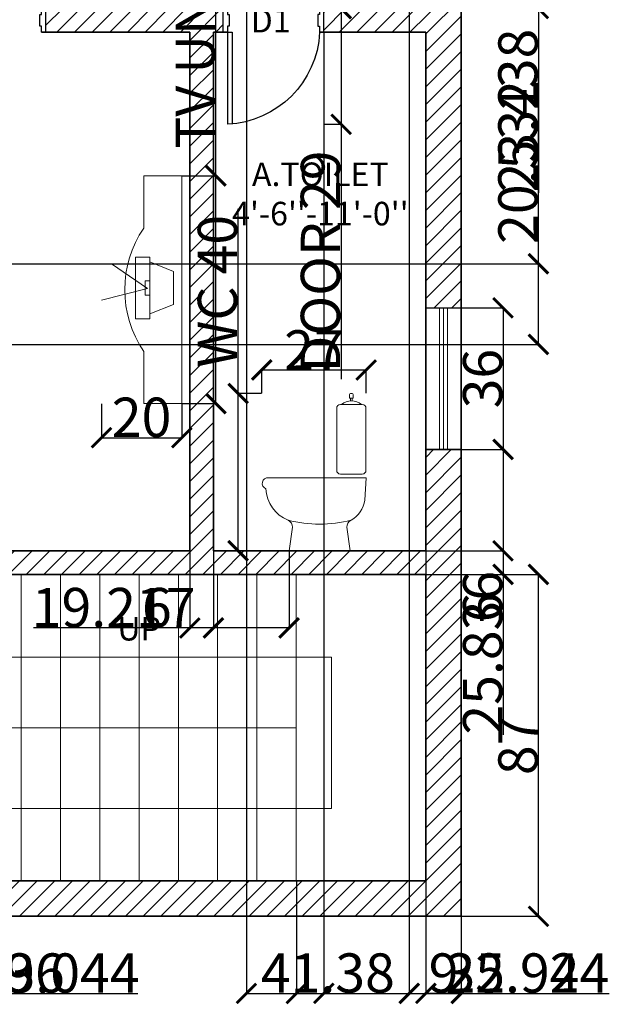
# Model space of a CAD drawing. Units: inches. Extents: x 90933 to 91345, y 21207 to 21646.
# Tile 2 of 4: x 91195 to 91345, y 21207 to 21458. Entities that reach past the tile are written whole.
import ezdxf

# ---------------------------------------------------------------- set-up
doc = ezdxf.new("R2010")
doc.units = ezdxf.units.IN
for name, color, linetype, lineweight in [('A-ANNO-DIMS', 2, 'Continuous', 18), ('A-ANNO-TEXT', 7, 'Continuous', 18), ('A-AREA-IDEN', 7, 'Continuous', 25), ('A-FLOR-FIXT', 9, 'Continuous', 18), ('A-WALL-PATT', 8, 'Continuous', 13), ('B-FURNITURE', 9, 'Continuous', 18), ('Doors', 34, 'Continuous', 25), ('Steps', 50, 'Continuous', 18), ('Ven', 120, 'Continuous', 18), ('Walls', 7, 'Continuous', 35)]:
    doc.layers.add(name, color=color, linetype=linetype, lineweight=lineweight)
doc.styles.get("Standard").update_dxf_attribs({"font": 'arial.ttf'})
doc.dimstyles.get("Standard").update_dxf_attribs({"dimtxt": 10, "dimasz": 5, "dimexe": 0.18, "dimexo": 0.0625, "dimgap": 0.09, "dimtad": 1, "dimdec": 1, "dimzin": 0, "dimdsep": 46, "dimlunit": 4, "dimtxsty": 'Standard', "dimblk": 'ARCHTICK', "dimcen": 0.09, "dimadec": 0, "dimazin": 0, "dimtfac": 1, "dimtdec": 1, "dimtofl": 0, "dimtmove": 0, "dimatfit": 3, "dimldrblk": 'NONE', "dimfxl": 1, "dimtolj": 1, "dimtzin": 0, "dimarcsym": 0})

# ---------------------------------------------------------------- blocks, each defined once
blk = doc.blocks.new('toil-el-1')
at = {"color": 0, "linetype": 'ByBlock'}
for p, q in [((-0.0048, 1.026), (-0.0048, 1.002)), ((-0.0048, 1.002), (0.0192, 1.002)), ((0.0012, 1.032), (0.0132, 1.032)), ((0.0012, 1.002), (0.0012, 0.984)), ((0.0132, 1.002), (0.0132, 0.984)), ((0.0192, 1.026), (0.0192, 1.002)), ((-0.0888, 0.936), (-0.0888, 0.528)), ((0.0792, 0.96), (-0.0648, 0.96)), ((0.1032, 0.936), (0.1032, 0.528)), ((0.1047, 0.48), (-0.543, 0.48)), ((0.0792, 0.504), (-0.0648, 0.504)), ((0.0966, 0.3327), (0.1047, 0.48)), ((-0.3785, 0.1552), (-0.4013, 0)), ((-0.0228, 0.1552), (0, 0)), ((-0.4013, 0), (0, 0))]:
    blk.add_line(p, q, dxfattribs=at)
for centre, radius, start, end in [((0.0084, 0.8817), 0.1023, 49.95059, 130.04941), ((0.0012, 1.026), 0.006, 90, 180), ((0.0132, 1.026), 0.006, 0, 90), ((-0.0648, 0.936), 0.024, 90, 180), ((0.0792, 0.936), 0.024, 0, 90), ((-0.0648, 0.528), 0.024, 180, 270), ((0.0792, 0.528), 0.024, 270, 0), ((-0.5394, 0.4428), 0.0373, 84.42239, 249.75453), ((-0.3163, 0.4187), 0.2362, 182.64484, 247.30718), ((-0.0919, 0.3648), 0.1912, 300.87439, 350.34418), ((-0.4257, 0.1572), 0.0472, 357.60433, 67.30718), ((-0.2006, 1.0367), 0.8612, 256.10247, 283.89753), ((0.0244, 0.1572), 0.0472, 112.69282, 182.39567)]:
    blk.add_arc(centre, radius, start, end, dxfattribs=at)
blk = doc.blocks.new('AP0B05')
for p, q in [((35, 100), (35, 880)), ((75, 100), (75, 878.9))]:
    blk.add_line(p, q)
for points in [[(0, 100), (0, -100), (35, -100), (35, -50), (50, -50), (50, 50), (35, 50), (35, 100)], [(850, 100), (850, -100), (815, -100), (815, -50), (800, -50), (800, 50), (815, 50), (815, 100)]]:
    blk.add_lwpolyline(points, close=True)
blk.add_lwpolyline([(35, 100), (75, 100)])
blk.add_arc((-2.4, 62.6), 818.3, 2.62122, 87.37878)
blk = doc.blocks.new('banghe81')
for p, q in [((-500, 3000), (0, 3000)), ((-500, 2312), (-500, 3000)), ((0, 3000), (0, 0)), ((-925, 1843), (-450, 1517)), ((-607, 1930), (-419, 1930)), ((-607, 1117), (-607, 1930)), ((-419, 1930), (-419, 1117)), ((-107, 1742), (-419, 1867)), ((-107, 1305), (-107, 1742)), ((-482, 1617), (-482, 1430)), ((-419, 1617), (-482, 1617)), ((-450, 1517), (-1057, 1361)), ((-482, 1430), (-419, 1430)), ((-419, 1180), (-107, 1305)), ((-419, 1117), (-607, 1117)), ((-500, 0), (-500, 688)), ((0, 0), (-500, 0)), ((-500, 0), (-500, 0))]:
    blk.add_line(p, q)
blk.add_arc((695, 1500), 1445, 145.7945, 214.2055)
blk = doc.blocks.new('_ArchTick')
at = {"color": 0, "linetype": 'ByBlock', "const_width": 0.15}
blk.add_lwpolyline([(-0.5, -0.5), (0.5, 0.5)], dxfattribs=at)
blk = doc.blocks.new('*D22')
at = {"layer": 'A-ANNO-DIMS', "color": 0, "lineweight": -2, "transparency": 16777216}
for p, q in [((91272.22, 21460.62), (91276.76, 21460.62)), ((91276.58, 21460.62), (91276.58, 21431.16)), ((91272.22, 21431.16), (91276.76, 21431.16)), ((91276.58, 21431.16), (91276.58, 21366.34))]:
    blk.add_line(p, q, dxfattribs=at)
at = {"layer": 'Defpoints', "color": 0, "transparency": 16777216}
for p in [(91272.16, 21460.62), (91272.16, 21431.16), (91276.58, 21431.16)]:
    blk.add_point(p, dxfattribs=at)
at = {"layer": 'A-ANNO-DIMS', "color": 0, "lineweight": -2, "transparency": 16777216, "xscale": 5, "yscale": 5, "zscale": 5}
for p, rotation in [((91276.58, 21460.62), 90), ((91276.58, 21431.16), 270)]:
    blk.add_blockref('_ArchTick', p, dxfattribs=dict(at, rotation=rotation))
at = {"layer": 'A-ANNO-DIMS', "color": 0, "transparency": 16777216, "insert": (91271.31, 21396.25), "char_height": 10, "attachment_point": 5, "rotation": 90}
blk.add_mtext('\\A1;DOOR 29', dxfattribs=at)
blk = doc.blocks.new('_None')
blk = doc.blocks.new('*D32')
at = {"layer": 'A-ANNO-DIMS', "color": 0, "lineweight": -2, "transparency": 16777216}
for p, q in [((91250.38, 21362.65), (91250.38, 21409.68)), ((91256.32, 21362.65), (91250.2, 21362.65)), ((91250.38, 21322.62), (91250.38, 21362.65)), ((91256.32, 21322.62), (91250.2, 21322.62))]:
    blk.add_line(p, q, dxfattribs=at)
at = {"layer": 'Defpoints', "color": 0, "transparency": 16777216}
for p in [(91250.38, 21362.65), (91256.38, 21362.65), (91256.38, 21322.62)]:
    blk.add_point(p, dxfattribs=at)
at = {"layer": 'A-ANNO-DIMS', "color": 0, "lineweight": -2, "transparency": 16777216, "xscale": 5, "yscale": 5, "zscale": 5}
for p, rotation in [((91250.38, 21362.65), 90), ((91250.38, 21322.62), 270)]:
    blk.add_blockref('_ArchTick', p, dxfattribs=dict(at, rotation=rotation))
at = {"layer": 'A-ANNO-DIMS', "color": 0, "transparency": 16777216, "insert": (91245.12, 21388.67), "char_height": 10, "attachment_point": 5, "rotation": 90}
blk.add_mtext('\\A1;WC 40', dxfattribs=at)
blk = doc.blocks.new('*D33')
at = {"layer": 'A-ANNO-DIMS', "color": 0, "lineweight": -2, "transparency": 16777216}
for p, q in [((91256.38, 21362.71), (91256.38, 21368.83)), ((91256.38, 21368.65), (91282.95, 21368.65)), ((91282.95, 21362.71), (91282.95, 21368.83))]:
    blk.add_line(p, q, dxfattribs=at)
at = {"layer": 'Defpoints', "color": 0, "transparency": 16777216}
for p in [(91282.95, 21368.65), (91256.38, 21362.65), (91282.95, 21362.65)]:
    blk.add_point(p, dxfattribs=at)
at = {"layer": 'A-ANNO-DIMS', "color": 0, "lineweight": -2, "transparency": 16777216, "xscale": 5, "yscale": 5, "zscale": 5, "rotation": 180}
blk.add_blockref('_ArchTick', (91256.38, 21368.65), dxfattribs=at)
at = {"layer": 'A-ANNO-DIMS', "color": 0, "lineweight": -2, "transparency": 16777216, "xscale": 5, "yscale": 5, "zscale": 5}
blk.add_blockref('_ArchTick', (91282.95, 21368.65), dxfattribs=at)
at = {"layer": 'A-ANNO-DIMS', "color": 0, "transparency": 16777216, "insert": (91269.66, 21373.76), "char_height": 10, "attachment_point": 5}
blk.add_mtext('\\A1;27', dxfattribs=at)
blk = doc.blocks.new('*D36')
at = {"layer": 'A-ANNO-DIMS', "color": 0, "lineweight": -2, "transparency": 16777216}
for p, q in [((91244.73, 21418.04), (91244.73, 21496.03)), ((91236.1, 21418.04), (91244.91, 21418.04)), ((91244.73, 21360.1), (91244.73, 21418.04)), ((91236.1, 21360.1), (91244.91, 21360.1))]:
    blk.add_line(p, q, dxfattribs=at)
at = {"layer": 'Defpoints', "color": 0, "transparency": 16777216}
for p in [(91236.04, 21418.04), (91244.73, 21418.04), (91236.04, 21360.1)]:
    blk.add_point(p, dxfattribs=at)
at = {"layer": 'A-ANNO-DIMS', "color": 0, "lineweight": -2, "transparency": 16777216, "xscale": 5, "yscale": 5, "zscale": 5}
for p, rotation in [((91244.73, 21418.04), 90), ((91244.73, 21360.1), 270)]:
    blk.add_blockref('_ArchTick', p, dxfattribs=dict(at, rotation=rotation))
at = {"layer": 'A-ANNO-DIMS', "color": 0, "transparency": 16777216, "insert": (91239.53, 21459.53), "char_height": 10, "attachment_point": 5, "rotation": 90}
blk.add_mtext('\\A1;TV UNIT 58', dxfattribs=at)
blk = doc.blocks.new('*D37')
at = {"layer": 'A-ANNO-DIMS', "color": 0, "lineweight": -2, "transparency": 16777216}
for p, q in [((91215.62, 21360.04), (91215.62, 21351.23)), ((91236.04, 21360.04), (91236.04, 21351.23)), ((91215.62, 21351.41), (91236.04, 21351.41))]:
    blk.add_line(p, q, dxfattribs=at)
at = {"layer": 'Defpoints', "color": 0, "transparency": 16777216}
for p in [(91215.62, 21360.1), (91236.04, 21360.1), (91236.04, 21351.41)]:
    blk.add_point(p, dxfattribs=at)
at = {"layer": 'A-ANNO-DIMS', "color": 0, "lineweight": -2, "transparency": 16777216, "xscale": 5, "yscale": 5, "zscale": 5, "rotation": 180}
blk.add_blockref('_ArchTick', (91215.62, 21351.41), dxfattribs=at)
at = {"layer": 'A-ANNO-DIMS', "color": 0, "lineweight": -2, "transparency": 16777216, "xscale": 5, "yscale": 5, "zscale": 5}
blk.add_blockref('_ArchTick', (91236.04, 21351.41), dxfattribs=at)
at = {"layer": 'A-ANNO-DIMS', "color": 0, "transparency": 16777216, "insert": (91225.83, 21356.61), "char_height": 10, "attachment_point": 5}
blk.add_mtext('\\A1;20', dxfattribs=at)
blk = doc.blocks.new('*D39')
at = {"layer": 'A-ANNO-DIMS', "color": 0, "lineweight": -2, "transparency": 16777216}
for p, q in [((91298.16, 21348.45), (91317.91, 21348.45)), ((91317.73, 21348.45), (91317.73, 21322.62)), ((91298.16, 21322.62), (91317.91, 21322.62)), ((91317.73, 21322.62), (91317.73, 21275.76))]:
    blk.add_line(p, q, dxfattribs=at)
at = {"layer": 'Defpoints', "color": 0, "transparency": 16777216}
for p in [(91298.1, 21348.45), (91298.1, 21322.62), (91317.73, 21322.62)]:
    blk.add_point(p, dxfattribs=at)
at = {"layer": 'A-ANNO-DIMS', "color": 0, "lineweight": -2, "transparency": 16777216, "xscale": 5, "yscale": 5, "zscale": 5}
for p, rotation in [((91317.73, 21348.45), 90), ((91317.73, 21322.62), 270)]:
    blk.add_blockref('_ArchTick', p, dxfattribs=dict(at, rotation=rotation))
at = {"layer": 'A-ANNO-DIMS', "color": 0, "transparency": 16777216, "insert": (91312.53, 21296.69), "char_height": 10, "attachment_point": 5, "rotation": 90}
blk.add_mtext('\\A1;25.836', dxfattribs=at)
blk = doc.blocks.new('*D40')
at = {"layer": 'A-ANNO-DIMS', "color": 0, "lineweight": -2, "transparency": 16777216}
for p, q in [((91298.16, 21384.45), (91317.91, 21384.45)), ((91317.73, 21384.45), (91317.73, 21348.45)), ((91298.16, 21348.45), (91317.91, 21348.45))]:
    blk.add_line(p, q, dxfattribs=at)
at = {"layer": 'Defpoints', "color": 0, "transparency": 16777216}
for p in [(91298.1, 21384.45), (91298.1, 21348.45), (91317.73, 21348.45)]:
    blk.add_point(p, dxfattribs=at)
at = {"layer": 'A-ANNO-DIMS', "color": 0, "lineweight": -2, "transparency": 16777216, "xscale": 5, "yscale": 5, "zscale": 5}
for p, rotation in [((91317.73, 21384.45), 90), ((91317.73, 21348.45), 270)]:
    blk.add_blockref('_ArchTick', p, dxfattribs=dict(at, rotation=rotation))
at = {"layer": 'A-ANNO-DIMS', "color": 0, "transparency": 16777216, "insert": (91312.53, 21366.45), "char_height": 10, "attachment_point": 5, "rotation": 90}
blk.add_mtext('\\A1;36', dxfattribs=at)
blk = doc.blocks.new('*D41')
at = {"layer": 'A-ANNO-DIMS', "color": 0, "lineweight": -2, "transparency": 16777216}
for p, q in [((91166.1, 21592.55), (91166.1, 21209.81)), ((91179.14, 21592.55), (91179.14, 21209.81)), ((91166.1, 21209.99), (91179.14, 21209.99)), ((91179.14, 21209.99), (91224.86, 21209.99))]:
    blk.add_line(p, q, dxfattribs=at)
at = {"layer": 'Defpoints', "color": 0, "transparency": 16777216}
for p in [(91166.1, 21592.62), (91179.14, 21592.62), (91179.14, 21209.99)]:
    blk.add_point(p, dxfattribs=at)
at = {"layer": 'A-ANNO-DIMS', "color": 0, "lineweight": -2, "transparency": 16777216, "xscale": 5, "yscale": 5, "zscale": 5, "rotation": 180}
blk.add_blockref('_ArchTick', (91166.1, 21209.99), dxfattribs=at)
at = {"layer": 'A-ANNO-DIMS', "color": 0, "lineweight": -2, "transparency": 16777216, "xscale": 5, "yscale": 5, "zscale": 5}
blk.add_blockref('_ArchTick', (91179.14, 21209.99), dxfattribs=at)
at = {"layer": 'A-ANNO-DIMS', "color": 0, "transparency": 16777216, "insert": (91204.5, 21215.18), "char_height": 10, "attachment_point": 5}
blk.add_mtext('\\A1;13.044', dxfattribs=at)
blk = doc.blocks.new('*D49')
at = {"layer": 'A-ANNO-DIMS', "color": 0, "lineweight": -2, "transparency": 16777216}
for p, q in [((91160.1, 21460.55), (91160.1, 21209.81)), ((91142.5, 21454.55), (91142.5, 21209.81)), ((91142.5, 21209.99), (91160.1, 21209.99)), ((91160.1, 21209.99), (91205.85, 21209.99))]:
    blk.add_line(p, q, dxfattribs=at)
at = {"layer": 'Defpoints', "color": 0, "transparency": 16777216}
for p in [(91160.1, 21460.62), (91142.5, 21454.62), (91160.1, 21209.99)]:
    blk.add_point(p, dxfattribs=at)
at = {"layer": 'A-ANNO-DIMS', "color": 0, "lineweight": -2, "transparency": 16777216, "xscale": 5, "yscale": 5, "zscale": 5, "rotation": 180}
blk.add_blockref('_ArchTick', (91142.5, 21209.99), dxfattribs=at)
at = {"layer": 'A-ANNO-DIMS', "color": 0, "lineweight": -2, "transparency": 16777216, "xscale": 5, "yscale": 5, "zscale": 5}
blk.add_blockref('_ArchTick', (91160.1, 21209.99), dxfattribs=at)
at = {"layer": 'A-ANNO-DIMS', "color": 0, "transparency": 16777216, "insert": (91185.47, 21215.18), "char_height": 10, "attachment_point": 5}
blk.add_mtext('\\A1;17.596', dxfattribs=at)
blk = doc.blocks.new('*D51')
at = {"layer": 'A-ANNO-DIMS', "color": 0, "lineweight": -2, "transparency": 16777216}
for p, q in [((91272.16, 21454.54), (91272.16, 21209.81)), ((91298.1, 21454.55), (91298.1, 21209.81)), ((91272.16, 21209.99), (91298.1, 21209.99)), ((91298.1, 21209.99), (91337.15, 21209.99))]:
    blk.add_line(p, q, dxfattribs=at)
at = {"layer": 'Defpoints', "color": 0, "transparency": 16777216}
for p in [(91272.16, 21454.6), (91298.1, 21454.62), (91298.1, 21209.99)]:
    blk.add_point(p, dxfattribs=at)
at = {"layer": 'A-ANNO-DIMS', "color": 0, "lineweight": -2, "transparency": 16777216, "xscale": 5, "yscale": 5, "zscale": 5, "rotation": 180}
blk.add_blockref('_ArchTick', (91272.16, 21209.99), dxfattribs=at)
at = {"layer": 'A-ANNO-DIMS', "color": 0, "lineweight": -2, "transparency": 16777216, "xscale": 5, "yscale": 5, "zscale": 5}
blk.add_blockref('_ArchTick', (91298.1, 21209.99), dxfattribs=at)
at = {"layer": 'A-ANNO-DIMS', "color": 0, "transparency": 16777216, "insert": (91320.13, 21215.18), "char_height": 10, "attachment_point": 5}
blk.add_mtext('\\A1;25.94', dxfattribs=at)
blk = doc.blocks.new('*D54')
at = {"layer": 'A-ANNO-DIMS', "color": 0, "lineweight": -2, "transparency": 16777216}
for p, q in [((91298.1, 21238.55), (91298.1, 21209.81)), ((91307.1, 21229.55), (91307.1, 21209.81)), ((91307.1, 21209.99), (91298.1, 21209.99))]:
    blk.add_line(p, q, dxfattribs=at)
at = {"layer": 'Defpoints', "color": 0, "transparency": 16777216}
for p in [(91298.1, 21238.62), (91307.1, 21229.62), (91298.1, 21209.99)]:
    blk.add_point(p, dxfattribs=at)
at = {"layer": 'A-ANNO-DIMS', "color": 0, "lineweight": -2, "transparency": 16777216, "xscale": 5, "yscale": 5, "zscale": 5, "rotation": 180}
blk.add_blockref('_ArchTick', (91298.1, 21209.99), dxfattribs=at)
at = {"layer": 'A-ANNO-DIMS', "color": 0, "lineweight": -2, "transparency": 16777216, "xscale": 5, "yscale": 5, "zscale": 5}
blk.add_blockref('_ArchTick', (91307.1, 21209.99), dxfattribs=at)
at = {"layer": 'A-ANNO-DIMS', "color": 0, "transparency": 16777216, "insert": (91302.6, 21215.18), "char_height": 10, "attachment_point": 5}
blk.add_mtext('\\A1;9', dxfattribs=at)
blk = doc.blocks.new('*D56')
at = {"layer": 'A-ANNO-DIMS', "color": 0, "lineweight": -2, "transparency": 16777216}
for p, q in [((91265.18, 21238.55), (91265.18, 21209.81)), ((91298.1, 21238.55), (91298.1, 21209.81)), ((91265.18, 21209.99), (91298.1, 21209.99)), ((91298.1, 21209.99), (91344.75, 21209.99))]:
    blk.add_line(p, q, dxfattribs=at)
at = {"layer": 'Defpoints', "color": 0, "transparency": 16777216}
for p in [(91265.18, 21238.62), (91298.1, 21238.62), (91298.1, 21209.99)]:
    blk.add_point(p, dxfattribs=at)
at = {"layer": 'A-ANNO-DIMS', "color": 0, "lineweight": -2, "transparency": 16777216, "xscale": 5, "yscale": 5, "zscale": 5, "rotation": 180}
blk.add_blockref('_ArchTick', (91265.18, 21209.99), dxfattribs=at)
at = {"layer": 'A-ANNO-DIMS', "color": 0, "lineweight": -2, "transparency": 16777216, "xscale": 5, "yscale": 5, "zscale": 5}
blk.add_blockref('_ArchTick', (91298.1, 21209.99), dxfattribs=at)
at = {"layer": 'A-ANNO-DIMS', "color": 0, "transparency": 16777216, "insert": (91323.92, 21215.18), "char_height": 10, "attachment_point": 5}
blk.add_mtext('\\A1;32.924', dxfattribs=at)
blk = doc.blocks.new('*D61')
at = {"layer": 'A-ANNO-DIMS', "color": 0, "lineweight": -2, "transparency": 16777216}
for p, q in [((91326.73, 21395.68), (91326.73, 21442.44)), ((91153.57, 21395.68), (91326.91, 21395.68)), ((91326.73, 21375.15), (91326.73, 21395.68)), ((91153.57, 21375.15), (91326.91, 21375.15))]:
    blk.add_line(p, q, dxfattribs=at)
at = {"layer": 'Defpoints', "color": 0, "transparency": 16777216}
for p in [(91153.51, 21395.68), (91326.73, 21395.68), (91153.51, 21375.15)]:
    blk.add_point(p, dxfattribs=at)
at = {"layer": 'A-ANNO-DIMS', "color": 0, "lineweight": -2, "transparency": 16777216, "xscale": 5, "yscale": 5, "zscale": 5}
for p, rotation in [((91326.73, 21395.68), 90), ((91326.73, 21375.15), 270)]:
    blk.add_blockref('_ArchTick', p, dxfattribs=dict(at, rotation=rotation))
at = {"layer": 'A-ANNO-DIMS', "color": 0, "transparency": 16777216, "insert": (91321.53, 21421.56), "char_height": 10, "attachment_point": 5, "rotation": 90}
blk.add_mtext('\\A1;20.532', dxfattribs=at)
blk = doc.blocks.new('*D62')
at = {"layer": 'A-ANNO-DIMS', "color": 0, "lineweight": -2, "transparency": 16777216}
for p, q in [((91252.49, 21576.95), (91252.49, 21209.81)), ((91293.88, 21576.95), (91293.88, 21209.81)), ((91252.49, 21209.99), (91293.88, 21209.99))]:
    blk.add_line(p, q, dxfattribs=at)
at = {"layer": 'Defpoints', "color": 0, "transparency": 16777216}
for p in [(91252.49, 21577.01), (91293.88, 21577.01), (91293.88, 21209.99)]:
    blk.add_point(p, dxfattribs=at)
at = {"layer": 'A-ANNO-DIMS', "color": 0, "lineweight": -2, "transparency": 16777216, "xscale": 5, "yscale": 5, "zscale": 5, "rotation": 180}
blk.add_blockref('_ArchTick', (91252.49, 21209.99), dxfattribs=at)
at = {"layer": 'A-ANNO-DIMS', "color": 0, "lineweight": -2, "transparency": 16777216, "xscale": 5, "yscale": 5, "zscale": 5}
blk.add_blockref('_ArchTick', (91293.88, 21209.99), dxfattribs=at)
at = {"layer": 'A-ANNO-DIMS', "color": 0, "transparency": 16777216, "insert": (91273.18, 21215.18), "char_height": 10, "attachment_point": 5}
blk.add_mtext('\\A1;41.38', dxfattribs=at)
blk = doc.blocks.new('*D68')
at = {"layer": 'A-ANNO-DIMS', "color": 0, "lineweight": -2, "transparency": 16777216}
for p, q in [((91296.1, 21484.05), (91326.91, 21484.05)), ((91326.73, 21484.05), (91326.73, 21460.62)), ((91298.16, 21460.62), (91326.91, 21460.62)), ((91326.73, 21460.62), (91326.73, 21413.73))]:
    blk.add_line(p, q, dxfattribs=at)
at = {"layer": 'Defpoints', "color": 0, "transparency": 16777216}
for p in [(91296.04, 21484.05), (91298.1, 21460.62), (91326.73, 21460.62)]:
    blk.add_point(p, dxfattribs=at)
at = {"layer": 'A-ANNO-DIMS', "color": 0, "lineweight": -2, "transparency": 16777216, "xscale": 5, "yscale": 5, "zscale": 5}
for p, rotation in [((91326.73, 21484.05), 90), ((91326.73, 21460.62), 270)]:
    blk.add_blockref('_ArchTick', p, dxfattribs=dict(at, rotation=rotation))
at = {"layer": 'A-ANNO-DIMS', "color": 0, "transparency": 16777216, "insert": (91321.53, 21434.67), "char_height": 10, "attachment_point": 5, "rotation": 90}
blk.add_mtext('\\A1;23.438', dxfattribs=at)
blk = doc.blocks.new('*D69')
at = {"layer": 'A-ANNO-DIMS', "color": 0, "lineweight": -2, "transparency": 16777216}
for p, q in [((91244.1, 21322.55), (91244.1, 21302.81)), ((91263.32, 21322.55), (91263.32, 21302.81)), ((91244.1, 21302.99), (91198.35, 21302.99)), ((91263.32, 21302.99), (91244.1, 21302.99))]:
    blk.add_line(p, q, dxfattribs=at)
at = {"layer": 'Defpoints', "color": 0, "transparency": 16777216}
for p in [(91244.1, 21322.62), (91263.32, 21322.62), (91244.1, 21302.99)]:
    blk.add_point(p, dxfattribs=at)
at = {"layer": 'A-ANNO-DIMS', "color": 0, "lineweight": -2, "transparency": 16777216, "xscale": 5, "yscale": 5, "zscale": 5, "rotation": 180}
blk.add_blockref('_ArchTick', (91244.1, 21302.99), dxfattribs=at)
at = {"layer": 'A-ANNO-DIMS', "color": 0, "lineweight": -2, "transparency": 16777216, "xscale": 5, "yscale": 5, "zscale": 5}
blk.add_blockref('_ArchTick', (91263.32, 21302.99), dxfattribs=at)
at = {"layer": 'A-ANNO-DIMS', "color": 0, "transparency": 16777216, "insert": (91218.72, 21308.18), "char_height": 10, "attachment_point": 5}
blk.add_mtext('\\A1;19.217', dxfattribs=at)
blk = doc.blocks.new('*D75')
at = {"layer": 'A-ANNO-DIMS', "color": 0, "lineweight": -2, "transparency": 16777216}
for p, q in [((91298.16, 21316.62), (91326.91, 21316.62)), ((91326.73, 21229.62), (91326.73, 21316.62)), ((91307.16, 21229.62), (91326.91, 21229.62))]:
    blk.add_line(p, q, dxfattribs=at)
at = {"layer": 'Defpoints', "color": 0, "transparency": 16777216}
for p in [(91298.1, 21316.62), (91326.73, 21316.62), (91307.1, 21229.62)]:
    blk.add_point(p, dxfattribs=at)
at = {"layer": 'A-ANNO-DIMS', "color": 0, "lineweight": -2, "transparency": 16777216, "xscale": 5, "yscale": 5, "zscale": 5}
for p, rotation in [((91326.73, 21316.62), 90), ((91326.73, 21229.62), 270)]:
    blk.add_blockref('_ArchTick', p, dxfattribs=dict(at, rotation=rotation))
at = {"layer": 'A-ANNO-DIMS', "color": 0, "transparency": 16777216, "insert": (91321.53, 21273.12), "char_height": 10, "attachment_point": 5, "rotation": 90}
blk.add_mtext('\\A1;87', dxfattribs=at)
blk = doc.blocks.new('*D76')
at = {"layer": 'A-ANNO-DIMS', "color": 0, "lineweight": -2, "transparency": 16777216}
for p, q in [((91298.16, 21322.62), (91317.91, 21322.62)), ((91317.73, 21322.62), (91317.73, 21316.62)), ((91298.16, 21316.62), (91317.91, 21316.62)), ((91317.73, 21316.62), (91317.73, 21304.83))]:
    blk.add_line(p, q, dxfattribs=at)
at = {"layer": 'Defpoints', "color": 0, "transparency": 16777216}
for p in [(91298.1, 21322.62), (91298.1, 21316.62), (91317.73, 21316.62)]:
    blk.add_point(p, dxfattribs=at)
at = {"layer": 'A-ANNO-DIMS', "color": 0, "lineweight": -2, "transparency": 16777216, "xscale": 5, "yscale": 5, "zscale": 5}
for p, rotation in [((91317.73, 21322.62), 90), ((91317.73, 21316.62), 270)]:
    blk.add_blockref('_ArchTick', p, dxfattribs=dict(at, rotation=rotation))
at = {"layer": 'A-ANNO-DIMS', "color": 0, "transparency": 16777216, "insert": (91312.53, 21308.22), "char_height": 10, "attachment_point": 5, "rotation": 90}
blk.add_mtext('\\A1;6', dxfattribs=at)
blk = doc.blocks.new('*D77')
at = {"layer": 'A-ANNO-DIMS', "color": 0, "lineweight": -2, "transparency": 16777216}
for p, q in [((91238.1, 21322.55), (91238.1, 21302.81)), ((91244.1, 21322.55), (91244.1, 21302.81)), ((91238.1, 21302.99), (91226.32, 21302.99)), ((91244.1, 21302.99), (91238.1, 21302.99))]:
    blk.add_line(p, q, dxfattribs=at)
at = {"layer": 'Defpoints', "color": 0, "transparency": 16777216}
for p in [(91238.1, 21322.62), (91244.1, 21322.62), (91238.1, 21302.99)]:
    blk.add_point(p, dxfattribs=at)
at = {"layer": 'A-ANNO-DIMS', "color": 0, "lineweight": -2, "transparency": 16777216, "xscale": 5, "yscale": 5, "zscale": 5, "rotation": 180}
blk.add_blockref('_ArchTick', (91238.1, 21302.99), dxfattribs=at)
at = {"layer": 'A-ANNO-DIMS', "color": 0, "lineweight": -2, "transparency": 16777216, "xscale": 5, "yscale": 5, "zscale": 5}
blk.add_blockref('_ArchTick', (91244.1, 21302.99), dxfattribs=at)
at = {"layer": 'A-ANNO-DIMS', "color": 0, "transparency": 16777216, "insert": (91229.71, 21308.18), "char_height": 10, "attachment_point": 5}
blk.add_mtext('\\A1;6', dxfattribs=at)

msp = doc.modelspace()

# ---------------------------------------------------------------- hatches: boundary and pattern name
at = {"layer": 'A-WALL-PATT', "transparency": 33554585}
h = msp.add_hatch(dxfattribs=at)
h.set_pattern_fill('ANSI31', color=256)
h.paths.add_polyline_path([(91179.1445, 21601.6157), (91028.1004, 21601.6157), (91028.1004, 21515.2814), (91037.1004, 21515.2814), (91037.1004, 21592.6157), (91160.1004, 21592.6157), (91160.1004, 21460.6157), (91142.5048, 21460.6157), (91142.5048, 21454.6157), (91175.976, 21454.6157), (91175.976, 21460.6157), (91166.1004, 21460.6157), (91166.1004, 21592.6157), (91179.1445, 21592.6157)])
h.paths.add_polyline_path([(91307.1004, 21601.6157), (91215.1445, 21601.6157), (91215.1445, 21592.6157), (91298.1004, 21592.6157), (91298.1004, 21460.6157), (91272.1605, 21460.6157), (91272.1605, 21454.6157), (91298.1004, 21454.6157), (91298.1004, 21384.4519), (91307.1004, 21384.4519)])
h.paths.add_polyline_path([(91037.1004, 21454.6157), (91086.5447, 21454.6157), (91086.5447, 21460.6157), (91037.1004, 21460.6157), (91037.1004, 21479.2814), (91028.1004, 21479.2814), (91028.1004, 21412.6157), (91037.1004, 21412.6157)])
h.paths.add_polyline_path([(91307.1004, 21348.4519), (91298.1004, 21348.4519), (91298.1004, 21322.6157), (91244.1004, 21322.6157), (91244.1004, 21454.6157), (91246.6116, 21454.6157), (91246.6116, 21460.6157), (91201.4342, 21460.6157), (91201.4342, 21454.6157), (91238.1004, 21454.6157), (91238.1004, 21322.6157), (91160.7949, 21322.6157), (91160.7949, 21316.6157), (91298.1004, 21316.6157), (91298.1004, 21238.6157), (91160.1004, 21238.6157), (91160.1004, 21229.6157), (91307.1004, 21229.6157)])
h.paths.add_polyline_path([(91037.1004, 21316.6157), (91049.0004, 21316.6157), (91049.0004, 21322.6157), (91037.1004, 21322.6157), (91037.1004, 21364.6157), (91028.1004, 21364.6157), (91028.1004, 21229.6157), (91037.1004, 21229.6157)])
h.paths.add_polyline_path([(91112.7949, 21322.6157), (91074.4445, 21322.6157), (91074.4445, 21316.6157), (91112.7949, 21316.6157)])

# ---------------------------------------------------------------- linework, layer by layer
at = {"layer": 'Steps'}
for p, q in [((91195.1761, 21238.6157), (91195.1761, 21316.6157)), ((91205.1761, 21238.6157), (91205.1761, 21316.6157)), ((91215.1761, 21238.6157), (91215.1761, 21316.6157)), ((91225.1761, 21238.6157), (91225.1761, 21316.6157)), ((91235.1761, 21238.6157), (91235.1761, 21316.6157)), ((91245.1761, 21238.6157), (91245.1761, 21316.6157)), ((91255.1761, 21238.6157), (91255.1761, 21316.6157)), ((91265.1761, 21238.6157), (91265.1761, 21316.6157)), ((91165.1761, 21277.6157), (91265.1761, 21277.6157))]:
    msp.add_line(p, q, dxfattribs=at)
msp.add_lwpolyline([(91175.1761, 21257.0619), (91274.1452, 21257.0619), (91274.1452, 21295.5267), (91165.1761, 21295.5267)], dxfattribs=at)
at = {"layer": 'Ven'}
for p, q in [((91301.6004, 21348.4519), (91301.6004, 21384.4519)), ((91302.6004, 21348.4519), (91302.6004, 21384.4519)), ((91303.6004, 21348.4519), (91303.6004, 21384.4519))]:
    msp.add_line(p, q, dxfattribs=at)
msp.add_lwpolyline([(91298.1004, 21348.4519), (91298.1004, 21384.4519), (91307.1004, 21384.4519), (91307.1004, 21348.4519)], close=True, dxfattribs=at)
at = {"layer": 'Walls'}
for p, q in [((91307.1004, 21601.6157), (91307.1004, 21229.6157)), ((91200.3859, 21454.6157), (91238.1004, 21454.6157)), ((91238.1004, 21454.6157), (91238.1004, 21322.6157)), ((91244.1004, 21454.6157), (91244.1004, 21322.6157)), ((91244.1004, 21454.6157), (91247.6636, 21454.6157)), ((91271.1085, 21454.6157), (91298.1004, 21454.6157)), ((91298.1004, 21454.6157), (91298.1004, 21322.6157)), ((91073.3962, 21322.6157), (91238.1004, 21322.6157)), ((91244.1004, 21322.6157), (91298.1004, 21322.6157)), ((91073.3968, 21316.6157), (91298.1004, 21316.6157)), ((91298.1004, 21316.6157), (91298.1004, 21238.6157)), ((91160.1004, 21238.6157), (91298.1004, 21238.6157)), ((91160.1004, 21229.6157), (91307.1004, 21229.6157))]:
    msp.add_line(p, q, dxfattribs=at)

# ---------------------------------------------------------------- block references
at = {"layer": 'A-FLOR-FIXT', "xscale": 38.79146540525677, "yscale": 38.79146540525677, "zscale": 38.79146540525677}
msp.add_blockref('toil-el-1', (91278.8835, 21322.6157), dxfattribs=at)
at = {"layer": 'B-FURNITURE', "xscale": 0.0193128306136408, "yscale": 0.0193128306136408, "zscale": 0.0193128306136408}
msp.add_blockref('banghe81', (91236.0368, 21360.1043), dxfattribs=at)
at = {"layer": 'Doors', "xscale": 0.0299507821919959, "yscale": 0.0299507821919959, "zscale": 0.0299507821919959}
msp.add_blockref('AP0B05', (91175.976, 21457.6107), dxfattribs=at)
at = {"layer": 'Doors', "xscale": -0.0300575518172249, "yscale": 0.0300575518172249, "zscale": 0.0300575518172249, "rotation": 180}
msp.add_blockref('AP0B05', (91246.6116, 21457.6099), dxfattribs=at)

# ---------------------------------------------------------------- texts
at = {"layer": 'A-ANNO-TEXT'}
for s, p in [('D1', (91253.5575, 21454.5376)), ('UP', (91219.6606, 21299.8023))]:
    msp.add_text(s, height=6, dxfattribs=at).set_placement(p)
at = {"layer": 'A-AREA-IDEN', "insert": (91248.1976, 21421.4371), "char_height": 6, "attachment_point": 1}
msp.add_mtext_dynamic_manual_height_columns("\\pxqc;A.TOILET\\P4'-6''-11'-0''", width=46.179351, gutter_width=12.5, heights=[0], dxfattribs=at)

# ---------------------------------------------------------------- dimensions: what is measured, and where the dimension line sits
at = {"layer": 'A-ANNO-DIMS'}
for base, p1, p2, override, picture, middle in [((91179.1445, 21209.9857), (91166.1004, 21592.6157), (91179.1445, 21592.6157), {"dimdec": 3, "dimlfac": 1, "dimrnd": 0, "dimzin": 0, "dimdsep": 46, "dimlunit": 2}, '*D41', (91204.5006, 21215.1848)), ((91293.8759, 21209.9857), (91252.4937, 21577.015), (91293.8759, 21577.015), {"dimdec": 2, "dimlfac": 1, "dimrnd": 0, "dimzin": 0, "dimdsep": 46, "dimlunit": 2}, '*D62', (91273.1848, 21215.1848)), ((91160.1004, 21209.9857), (91142.5048, 21454.6157), (91160.1004, 21460.6157), {"dimdec": 3, "dimlfac": 1, "dimrnd": 0, "dimzin": 0, "dimdsep": 46, "dimlunit": 2}, '*D49', (91185.4735, 21215.1814)), ((91298.1004, 21209.9857), (91272.1605, 21454.6041), (91298.1004, 21454.6157), {"dimdec": 2, "dimlfac": 1, "dimrnd": 0, "dimzin": 0, "dimdsep": 46, "dimlunit": 2}, '*D51', (91320.1277, 21215.1814)), ((91282.9453, 21368.6534), (91256.3839, 21362.6485), (91282.9453, 21362.6485), {"dimdec": 0, "dimlfac": 1, "dimrnd": 0, "dimzin": 0, "dimdsep": 46, "dimlunit": 2}, '*D33', (91269.6646, 21373.7638)), ((91236.0368, 21351.4135), (91215.6215, 21360.1043), (91236.0368, 21360.1043), {"dimdec": 0, "dimlfac": 1, "dimrnd": 0, "dimzin": 0, "dimdsep": 46, "dimlunit": 2}, '*D37', (91225.8291, 21356.6092)), ((91298.1004, 21209.9857), (91265.1761, 21238.6157), (91298.1004, 21238.6157), {"dimdec": 3, "dimlfac": 1, "dimrnd": 0, "dimzin": 0, "dimdsep": 46, "dimlunit": 2}, '*D56', (91323.9237, 21215.1848)), ((91298.1004, 21209.9857), (91307.1004, 21229.6157), (91298.1004, 21238.6157), {"dimdec": 0, "dimlfac": 1, "dimrnd": 0, "dimzin": 0, "dimdsep": 46, "dimlunit": 2}, '*D54', (91302.6004, 21215.1814))]:
    dim = msp.add_linear_dim(base=base, p1=p1, p2=p2, dimstyle='Standard', override=override, dxfattribs=at)
    dim.commit()
    dim.dimension.update_dxf_attribs({"geometry": picture, "text_midpoint": middle})
for base, p1, p2, angle, text, picture, middle in [((91244.7276, 21418.0428), (91236.0368, 21360.1043), (91236.0368, 21418.0428), 90, 'TV UNIT <>', '*D36', (91239.5318, 21459.5345)), ((91276.5789, 21431.1593), (91272.1605, 21460.6157), (91272.1605, 21431.1593), 270, 'DOOR <>', '*D22', (91271.315, 21396.25)), ((91250.3789, 21362.6485), (91256.3839, 21322.6157), (91256.3839, 21362.6485), 90, 'WC <>', '*D32', (91245.1184, 21388.6661))]:
    dim = msp.add_linear_dim(base=base, p1=p1, p2=p2, angle=angle, text=text, dimstyle='Standard', override={"dimdec": 0, "dimlfac": 1, "dimrnd": 0, "dimzin": 0, "dimdsep": 46, "dimlunit": 2}, dxfattribs=at)
    dim.commit()
    dim.dimension.update_dxf_attribs({"geometry": picture, "text_midpoint": middle})
for base, p1, p2, angle, override, picture, middle in [((91326.73045, 21460.61566), (91296.0425, 21484.05324), (91298.10045, 21460.61566), 90, {"dimdec": 3, "dimlfac": 1, "dimrnd": 0, "dimzin": 0, "dimdsep": 46, "dimlunit": 2}, '*D68', (91321.53131, 21434.673)), ((91326.7305, 21395.6809), (91153.5083, 21375.1486), (91153.5083, 21395.6809), 90, {"dimdec": 3, "dimlfac": 1, "dimrnd": 0, "dimzin": 0, "dimdsep": 46, "dimlunit": 2}, '*D61', (91321.5313, 21421.5622)), ((91317.7305, 21348.4519), (91298.1004, 21384.4519), (91298.1004, 21348.4519), 270, {"dimdec": 0, "dimlfac": 1, "dimrnd": 0, "dimzin": 0, "dimdsep": 46, "dimlunit": 2}, '*D40', (91312.5313, 21366.4519)), ((91317.7305, 21322.6157), (91298.1004, 21348.4519), (91298.1004, 21322.6157), 270, {"dimdec": 3, "dimlfac": 1, "dimrnd": 0, "dimzin": 0, "dimdsep": 46, "dimlunit": 2}, '*D39', (91312.5313, 21296.6866)), ((91317.7305, 21316.6157), (91298.1004, 21322.6157), (91298.1004, 21316.6157), 270, {"dimdec": 0, "dimlfac": 1, "dimrnd": 0, "dimzin": 0, "dimdsep": 46, "dimlunit": 2}, '*D76', (91312.5347, 21308.2242)), ((91244.1004, 21302.9857), (91263.3174, 21322.6157), (91244.1004, 21322.6157), 180, {"dimdec": 3, "dimlfac": 1, "dimrnd": 0, "dimzin": 0, "dimdsep": 46, "dimlunit": 2}, '*D69', (91218.724, 21308.1814)), ((91238.1004, 21302.9857), (91244.1004, 21322.6157), (91238.1004, 21322.6157), 180, {"dimdec": 0, "dimlfac": 1, "dimrnd": 0, "dimzin": 0, "dimdsep": 46, "dimlunit": 2}, '*D77', (91229.7089, 21308.1814)), ((91326.7305, 21316.6157), (91307.1004, 21229.6157), (91298.1004, 21316.6157), 90, {"dimdec": 0, "dimlfac": 1, "dimrnd": 0, "dimzin": 0, "dimdsep": 46, "dimlunit": 2}, '*D75', (91321.5347, 21273.1157))]:
    dim = msp.add_linear_dim(base=base, p1=p1, p2=p2, angle=angle, dimstyle='Standard', override=override, dxfattribs=at)
    dim.commit()
    dim.dimension.update_dxf_attribs({"geometry": picture, "text_midpoint": middle})

doc.saveas('drawing.dxf')
